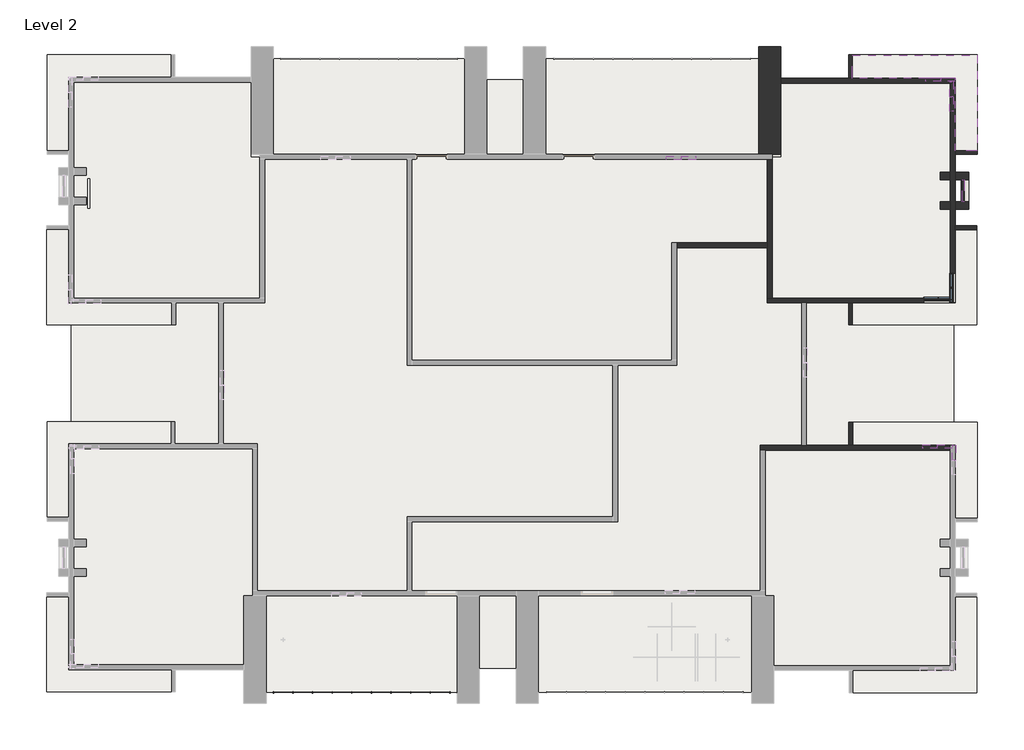
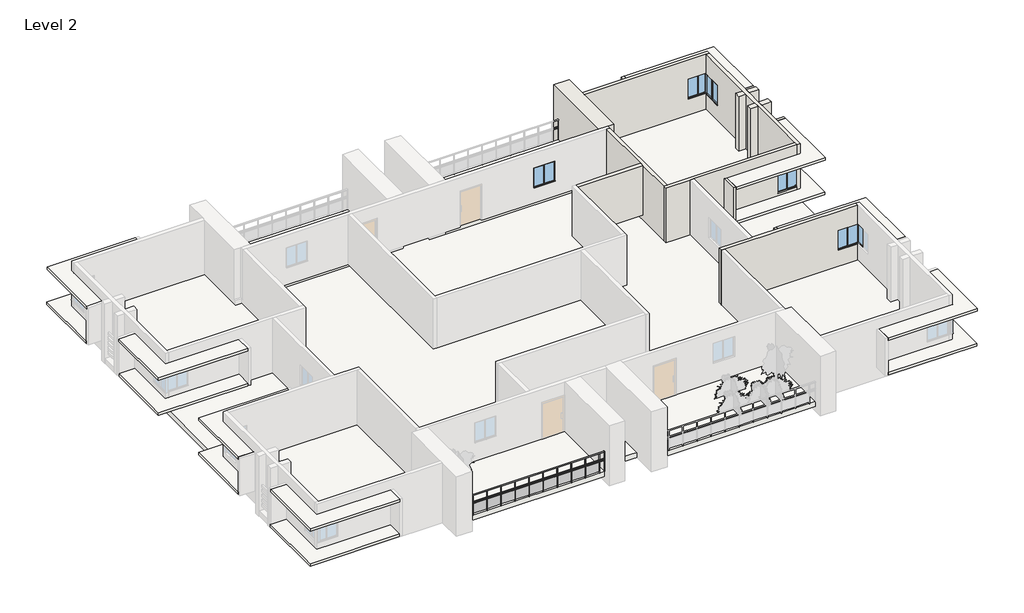
# One storey, part 3 of 4: 22 walls, 13 windows, 4 slabs, 1 railing.
"""IFC4 building model written with IfcOpenShell, lengths in millimetres."""

from ifc_helpers import new_model, si_unit, point, frame, origin, place, context, project, spatial, polyline, ellipse_curve, trimmed, outline, extrude, faceted_brep, transform, mapped, element, save
from ifc_brep_helpers import plane_surface, extruded_surface, advanced_brep
from components import window_20ff4747

model = new_model("IFC4")

# Units and contexts
model_context = context("Model", 3, world=origin())
ifc_project = project(units=[si_unit("LENGTHUNIT", "METRE", prefix="MILLI")], contexts=[model_context])

# Site, building, storey
site = spatial("IfcSite", under=ifc_project)
building = spatial("IfcBuilding", under=site)
storey = spatial("IfcBuildingStorey", under=building, Name="Level 2", Elevation=3048.0)

# Railing
placement = place(None, origin())
element("IfcRailing", 1, ObjectType="Glass Panel - Bottom Fill", at=placement, inside=storey, context=model_context, shape_type="SolidModel", body=[
    advanced_brep(
    [(-6704.9479335, -9342.282663, 4876.8), (-6704.9479335, -9418.482663, 4876.8), (1219.8520665, -9342.282663, 4876.8), (1219.8520665, -9418.482663, 4876.8)],
    [
        (0, 1, ellipse_curve(frame((-6704.9479335, -9380.382663, 4876.8), z_axis=(-1.0, 0.0, 0.0), x_axis=(0.0, -1.0, 0.0)), 38.1, 28.575)),
        (1, 0, ellipse_curve(frame((-6704.9479335, -9380.382663, 4876.8), z_axis=(-1.0, 0.0, 0.0), x_axis=(0.0, -1.0, 0.0)), 38.1, 28.575)),
        (2, 3, ellipse_curve(frame((1219.8520665, -9380.382663, 4876.8), z_axis=(1.0, 0.0, 0.0), x_axis=(0.0, -1.0, 0.0)), 38.1, 28.575)),
        (3, 2, ellipse_curve(frame((1219.8520665, -9380.382663, 4876.8), z_axis=(1.0, 0.0, 0.0), x_axis=(0.0, -1.0, 0.0)), 38.1, 28.575)),
        (0, 2),
        (3, 1),
    ],
    [
        plane_surface(frame((-6704.9479335, -9380.382663, 4876.8), z_axis=(-1.0, 0.0, 0.0), x_axis=(0.0, 1.0, 0.0))),
        plane_surface(frame((1219.8520665, -9380.382663, 4876.8), z_axis=(1.0, 0.0, 0.0), x_axis=(0.0, 1.0, 0.0))),
        extruded_surface(trimmed(ellipse_curve(frame((1219.8520665, -9380.382663, 4876.8), z_axis=(-1.0, 0.0, 0.0), x_axis=(0.0, -1.0, 0.0)), 38.1, 28.575), [point((1219.8520665, -9342.282663, 4876.8))], [point((1219.8520665, -9418.482663, 4876.8))], True, "CARTESIAN"), (-7924.799999999999, 0.0, 0.0), 7924.799999999999),
        extruded_surface(trimmed(ellipse_curve(frame((1219.8520665, -9380.382663, 4876.8), z_axis=(-1.0, 0.0, 0.0), x_axis=(0.0, -1.0, 0.0)), 38.1, 28.575), [point((1219.8520665, -9418.482663, 4876.8))], [point((1219.8520665, -9342.282663, 4876.8))], True, "CARTESIAN"), (-7924.799999999999, 0.0, 0.0), 7924.799999999999),
    ],
    [
        (0, [[1, 2]]),
        (1, [[3, 4]]),
        (2, [[-1, 5, -4, 6]]),
        (3, [[-2, -6, -3, -5]]),
    ],
),
    extrude(outline(polyline([(-6704.9479335, -9393.082663), (-6704.9479335, -9367.682663), (1219.8520665, -9367.682663), (1219.8520665, -9393.082663), (-6704.9479335, -9393.082663)])), frame((0.0, 0.0, 4457.7), z_axis=(0.0, 0.0, 1.0), x_axis=(1.0, 0.0, 0.0)), (0.0, 0.0, 1.0), 25.4),
    extrude(outline(polyline([(-6704.9479335, -9393.082663), (-6704.9479335, -9367.682663), (1219.8520665, -9367.682663), (1219.8520665, -9393.082663), (-6704.9479335, -9393.082663)])), frame((0.0, 0.0, 4356.1), z_axis=(0.0, 0.0, 1.0), x_axis=(1.0, 0.0, 0.0)), (0.0, 0.0, 1.0), 25.4),
    extrude(outline(polyline([(908.7020665, -9405.782663), (908.7020665, -9354.982663), (921.4020665, -9354.982663), (921.4020665, -9405.782663), (908.7020665, -9405.782663)])), frame((0.0, 0.0, 3657.6), z_axis=(0.0, 0.0, 1.0), x_axis=(1.0, 0.0, 0.0)), (0.0, 0.0, 1.0), 1190.4788223),
    extrude(outline(polyline([(102.2520665, -9373.847506), (915.0520665, -9373.847506), (915.0520665, -9380.197506), (102.2520665, -9380.197506), (102.2520665, -9373.847506)])), frame((0.0, 0.0, 3759.2), z_axis=(0.0, 0.0, 1.0), x_axis=(1.0, 0.0, 0.0)), (0.0, 0.0, 1.0), 596.9),
    extrude(outline(polyline([(95.9020665, -9405.782663), (95.9020665, -9354.982663), (108.6020665, -9354.982663), (108.6020665, -9405.782663), (95.9020665, -9405.782663)])), frame((0.0, 0.0, 3657.6), z_axis=(0.0, 0.0, 1.0), x_axis=(1.0, 0.0, 0.0)), (0.0, 0.0, 1.0), 1190.4788223),
    extrude(outline(polyline([(-710.5479335, -9373.847506), (102.2520665, -9373.847506), (102.2520665, -9380.197506), (-710.5479335, -9380.197506), (-710.5479335, -9373.847506)])), frame((0.0, 0.0, 3759.2), z_axis=(0.0, 0.0, 1.0), x_axis=(1.0, 0.0, 0.0)), (0.0, 0.0, 1.0), 596.9),
    extrude(outline(polyline([(-716.8979335, -9405.782663), (-716.8979335, -9354.982663), (-704.1979335, -9354.982663), (-704.1979335, -9405.782663), (-716.8979335, -9405.782663)])), frame((0.0, 0.0, 3657.6), z_axis=(0.0, 0.0, 1.0), x_axis=(1.0, 0.0, 0.0)), (0.0, 0.0, 1.0), 1190.4788223),
    extrude(outline(polyline([(-1523.3479335, -9373.847506), (-710.5479335, -9373.847506), (-710.5479335, -9380.197506), (-1523.3479335, -9380.197506), (-1523.3479335, -9373.847506)])), frame((0.0, 0.0, 3759.2), z_axis=(0.0, 0.0, 1.0), x_axis=(1.0, 0.0, 0.0)), (0.0, 0.0, 1.0), 596.9),
    extrude(outline(polyline([(-1529.6979335, -9405.782663), (-1529.6979335, -9354.982663), (-1516.9979335, -9354.982663), (-1516.9979335, -9405.782663), (-1529.6979335, -9405.782663)])), frame((0.0, 0.0, 3657.6), z_axis=(0.0, 0.0, 1.0), x_axis=(1.0, 0.0, 0.0)), (0.0, 0.0, 1.0), 1190.4788223),
    extrude(outline(polyline([(-2336.1479335, -9373.847506), (-1523.3479335, -9373.847506), (-1523.3479335, -9380.197506), (-2336.1479335, -9380.197506), (-2336.1479335, -9373.847506)])), frame((0.0, 0.0, 3759.2), z_axis=(0.0, 0.0, 1.0), x_axis=(1.0, 0.0, 0.0)), (0.0, 0.0, 1.0), 596.9),
    extrude(outline(polyline([(-2342.4979335, -9405.782663), (-2342.4979335, -9354.982663), (-2329.7979335, -9354.982663), (-2329.7979335, -9405.782663), (-2342.4979335, -9405.782663)])), frame((0.0, 0.0, 3657.6), z_axis=(0.0, 0.0, 1.0), x_axis=(1.0, 0.0, 0.0)), (0.0, 0.0, 1.0), 1190.4788223),
    extrude(outline(polyline([(-3148.9479335, -9373.847506), (-2336.1479335, -9373.847506), (-2336.1479335, -9380.197506), (-3148.9479335, -9380.197506), (-3148.9479335, -9373.847506)])), frame((0.0, 0.0, 3759.2), z_axis=(0.0, 0.0, 1.0), x_axis=(1.0, 0.0, 0.0)), (0.0, 0.0, 1.0), 596.9),
    extrude(outline(polyline([(-3155.2979335, -9405.782663), (-3155.2979335, -9354.982663), (-3142.5979335, -9354.982663), (-3142.5979335, -9405.782663), (-3155.2979335, -9405.782663)])), frame((0.0, 0.0, 3657.6), z_axis=(0.0, 0.0, 1.0), x_axis=(1.0, 0.0, 0.0)), (0.0, 0.0, 1.0), 1190.4788223),
    extrude(outline(polyline([(-3961.7479335, -9373.847506), (-3148.9479335, -9373.847506), (-3148.9479335, -9380.197506), (-3961.7479335, -9380.197506), (-3961.7479335, -9373.847506)])), frame((0.0, 0.0, 3759.2), z_axis=(0.0, 0.0, 1.0), x_axis=(1.0, 0.0, 0.0)), (0.0, 0.0, 1.0), 596.9),
    extrude(outline(polyline([(-3968.0979335, -9405.782663), (-3968.0979335, -9354.982663), (-3955.3979335, -9354.982663), (-3955.3979335, -9405.782663), (-3968.0979335, -9405.782663)])), frame((0.0, 0.0, 3657.6), z_axis=(0.0, 0.0, 1.0), x_axis=(1.0, 0.0, 0.0)), (0.0, 0.0, 1.0), 1190.4788223),
    extrude(outline(polyline([(-4774.5479335, -9373.847506), (-3961.7479335, -9373.847506), (-3961.7479335, -9380.197506), (-4774.5479335, -9380.197506), (-4774.5479335, -9373.847506)])), frame((0.0, 0.0, 3759.2), z_axis=(0.0, 0.0, 1.0), x_axis=(1.0, 0.0, 0.0)), (0.0, 0.0, 1.0), 596.9),
    extrude(outline(polyline([(-4780.8979335, -9405.782663), (-4780.8979335, -9354.982663), (-4768.1979335, -9354.982663), (-4768.1979335, -9405.782663), (-4780.8979335, -9405.782663)])), frame((0.0, 0.0, 3657.6), z_axis=(0.0, 0.0, 1.0), x_axis=(1.0, 0.0, 0.0)), (0.0, 0.0, 1.0), 1190.4788223),
    extrude(outline(polyline([(-5587.3479335, -9373.847506), (-4774.5479335, -9373.847506), (-4774.5479335, -9380.197506), (-5587.3479335, -9380.197506), (-5587.3479335, -9373.847506)])), frame((0.0, 0.0, 3759.2), z_axis=(0.0, 0.0, 1.0), x_axis=(1.0, 0.0, 0.0)), (0.0, 0.0, 1.0), 596.9),
    extrude(outline(polyline([(-5593.6979335, -9405.782663), (-5593.6979335, -9354.982663), (-5580.9979335, -9354.982663), (-5580.9979335, -9405.782663), (-5593.6979335, -9405.782663)])), frame((0.0, 0.0, 3657.6), z_axis=(0.0, 0.0, 1.0), x_axis=(1.0, 0.0, 0.0)), (0.0, 0.0, 1.0), 1190.4788223),
    extrude(outline(polyline([(-6400.1479335, -9373.847506), (-5587.3479335, -9373.847506), (-5587.3479335, -9380.197506), (-6400.1479335, -9380.197506), (-6400.1479335, -9373.847506)])), frame((0.0, 0.0, 3759.2), z_axis=(0.0, 0.0, 1.0), x_axis=(1.0, 0.0, 0.0)), (0.0, 0.0, 1.0), 596.9),
    extrude(outline(polyline([(-6406.4979335, -9405.782663), (-6406.4979335, -9354.982663), (-6393.7979335, -9354.982663), (-6393.7979335, -9405.782663), (-6406.4979335, -9405.782663)])), frame((0.0, 0.0, 3657.6), z_axis=(0.0, 0.0, 1.0), x_axis=(1.0, 0.0, 0.0)), (0.0, 0.0, 1.0), 1190.4788223),
    extrude(outline(polyline([(1207.1520665, -9389.907663), (1207.1520665, -9370.857663), (1226.2020665, -9370.857663), (1226.2020665, -9389.907663), (1207.1520665, -9389.907663)])), frame((0.0, 0.0, 3657.6), z_axis=(0.0, 0.0, 1.0), x_axis=(1.0, 0.0, 0.0)), (0.0, 0.0, 1.0), 1190.4788223),
    extrude(outline(polyline([(-6711.2979335, -9389.907663), (-6711.2979335, -9370.857663), (-6692.2479335, -9370.857663), (-6692.2479335, -9389.907663), (-6711.2979335, -9389.907663)])), frame((0.0, 0.0, 3657.6), z_axis=(0.0, 0.0, 1.0), x_axis=(1.0, 0.0, 0.0)), (0.0, 0.0, 1.0), 1190.4788223),
])

# Slabs
element("IfcSlab", 2, ObjectType="Generic - 2'", at=placement, inside=storey, context=model_context, shape_type="SweptSolid", body=[
    extrude(outline(polyline([(21793.8520665, 16006.5548886), (21793.8520665, -8377.4451114), (-14782.1479335, -8377.4451114), (-14782.1479335, 16006.5548886), (21793.8520665, 16006.5548886)])), frame((0.0, 0.0, 3048.0), z_axis=(0.0, 0.0, 1.0), x_axis=(1.0, 0.0, 0.0)), (0.0, 0.0, 1.0), 304.8),
])
element("IfcSlab", 3, ObjectType="Generic - 2' gray", at=placement, inside=storey, context=model_context, shape_type="SweptSolid", body=[
    extrude(outline(polyline([(13411.8520665, -5363.830811), (13411.8520665, -9380.382663), (4572.6520665, -9380.382663), (4572.6520665, -5363.830811), (13411.8520665, -5363.830811)])), frame((0.0, 0.0, 3352.8), z_axis=(0.0, 0.0, 1.0), x_axis=(1.0, 0.0, 0.0)), (0.0, 0.0, 1.0), 304.8),
    extrude(outline(polyline([(-6704.9479335, -5363.1461695), (1219.8520665, -5363.1461695), (1219.8520665, -9380.382663), (-6704.9479335, -9380.382663), (-6704.9479335, -5363.1461695)])), frame((0.0, 0.0, 3352.8), z_axis=(0.0, 0.0, 1.0), x_axis=(1.0, 0.0, 0.0)), (0.0, 0.0, 1.0), 304.8),
    extrude(outline(polyline([(13716.6520665, 12912.4705944), (4877.4520665, 12912.4705944), (4877.4520665, 16886.1559451), (13716.6520665, 16886.1559451), (13716.6520665, 12912.4705944)])), frame((0.0, 0.0, 3352.8), z_axis=(0.0, 0.0, 1.0), x_axis=(1.0, 0.0, 0.0)), (0.0, 0.0, 1.0), 304.8),
    extrude(outline(polyline([(-6400.1479335, 12912.4705944), (-6400.1479335, 16886.1559451), (1524.6520665, 16886.1559451), (1524.6520665, 12912.4705944), (-6400.1479335, 12912.4705944)])), frame((0.0, 0.0, 3352.8), z_axis=(0.0, 0.0, 1.0), x_axis=(1.0, 0.0, 0.0)), (0.0, 0.0, 1.0), 304.8),
])
element("IfcSlab", 4, ObjectType="Generic - 6\"", at=placement, inside=storey, context=model_context, shape_type="SweptSolid", body=[
    extrude(outline(polyline([(-10616.5479335, -9354.6604699), (-15798.1479335, -9354.6604699), (-15798.1479335, -5392.2604699), (-14883.7479335, -5392.2604699), (-14883.7479335, -8338.6604699), (-14883.7479335, -8440.2604699), (-10616.5479335, -8440.2604699), (-10616.5479335, -9354.6604699)])), frame((0.0, 0.0, 3810.0), z_axis=(0.0, 0.0, 1.0), x_axis=(1.0, 0.0, 0.0)), (0.0, 0.0, 1.0), 152.4),
    extrude(outline(polyline([(-10633.1034654, 1834.0395301), (-10633.1034654, 919.6395301), (-14883.7479335, 919.6395301), (-14883.7479335, -2128.3604699), (-15775.8097154, -2128.3604699), (-15775.8097154, 1834.0395301), (-10633.1034654, 1834.0395301)])), frame((0.0, 0.0, 3810.0), z_axis=(0.0, 0.0, 1.0), x_axis=(1.0, 0.0, 0.0)), (0.0, 0.0, 1.0), 152.4),
    extrude(outline(polyline([(-10616.5479335, 5846.5548886), (-15798.1479335, 5846.5548886), (-15798.1479335, 9808.9548886), (-14883.7479335, 9808.9548886), (-14883.7479335, 6862.5548886), (-14883.7479335, 6760.9548886), (-10616.5479335, 6760.9548886), (-10616.5479335, 5846.5548886)])), frame((0.0, 0.0, 3810.0), z_axis=(0.0, 0.0, 1.0), x_axis=(1.0, 0.0, 0.0)), (0.0, 0.0, 1.0), 152.4),
    extrude(outline(polyline([(-10633.1034654, 17035.2548886), (-10633.1034654, 16120.8548886), (-14883.7479335, 16120.8548886), (-14883.7479335, 13072.8548886), (-15775.8097154, 13072.8548886), (-15775.8097154, 17035.2548886), (-10633.1034654, 17035.2548886)])), frame((0.0, 0.0, 3810.0), z_axis=(0.0, 0.0, 1.0), x_axis=(1.0, 0.0, 0.0)), (0.0, 0.0, 1.0), 152.4),
    extrude(outline(polyline([(17590.1520665, 17035.2548886), (22771.7520665, 17035.2548886), (22771.7520665, 13072.8548886), (21857.3520665, 13072.8548886), (21857.3520665, 16019.2548886), (21857.3520665, 16070.0548886), (17590.1520665, 16070.0548886), (17590.1520665, 16120.8548886), (17590.1520665, 17035.2548886)])), frame((0.0, 0.0, 3810.0), z_axis=(0.0, 0.0, 1.0), x_axis=(1.0, 0.0, 0.0)), (0.0, 0.0, 1.0), 152.4),
    extrude(outline(polyline([(17606.7075984, 5846.5548886), (17606.7075984, 6760.9548886), (21857.3520665, 6760.9548886), (21857.3520665, 9808.9548886), (22749.4138484, 9808.9548886), (22749.4138484, 5846.5548886), (17606.7075984, 5846.5548886)])), frame((0.0, 0.0, 3810.0), z_axis=(0.0, 0.0, 1.0), x_axis=(1.0, 0.0, 0.0)), (0.0, 0.0, 1.0), 152.4),
    extrude(outline(polyline([(17590.1520665, 1807.9548886), (22771.7520665, 1807.9548886), (22771.7520665, -2154.4451114), (21857.3520665, -2154.4451114), (21857.3520665, 791.9548886), (21857.3520665, 893.5548886), (17590.1520665, 893.5548886), (17590.1520665, 1807.9548886)])), frame((0.0, 0.0, 3810.0), z_axis=(0.0, 0.0, 1.0), x_axis=(1.0, 0.0, 0.0)), (0.0, 0.0, 1.0), 152.4),
    extrude(outline(polyline([(17606.7075984, -9380.7451114), (17606.7075984, -8466.3451114), (21857.3520665, -8466.3451114), (21857.3520665, -5418.3451114), (22749.4138484, -5418.3451114), (22749.4138484, -9380.7451114), (17606.7075984, -9380.7451114)])), frame((0.0, 0.0, 3810.0), z_axis=(0.0, 0.0, 1.0), x_axis=(1.0, 0.0, 0.0)), (0.0, 0.0, 1.0), 152.4),
])
element("IfcSlab", 5, ObjectType="Generic - 6\"", at=placement, inside=storey, context=model_context, shape_type="SweptSolid", body=[
    extrude(outline(polyline([(-10617.0810044, -9363.7552779), (-15798.6810044, -9363.7552779), (-15798.6810044, -5401.3552779), (-14884.2810044, -5401.3552779), (-14884.2810044, -8347.7552779), (-14884.2810044, -8449.3552779), (-10617.0810044, -8449.3552779), (-10617.0810044, -9363.7552779)])), frame((0.0, 0.0, 5943.6), z_axis=(0.0, 0.0, 1.0), x_axis=(1.0, 0.0, 0.0)), (0.0, 0.0, 1.0), 152.4),
    extrude(outline(polyline([(-10633.6365363, 1824.9447221), (-10633.6365363, 910.5447221), (-14884.2810044, 910.5447221), (-14884.2810044, -2137.4552779), (-15776.3427863, -2137.4552779), (-15776.3427863, 1824.9447221), (-10633.6365363, 1824.9447221)])), frame((0.0, 0.0, 5943.6), z_axis=(0.0, 0.0, 1.0), x_axis=(1.0, 0.0, 0.0)), (0.0, 0.0, 1.0), 152.4),
    extrude(outline(polyline([(-10617.0810044, 5837.4600805), (-15798.6810044, 5837.4600805), (-15798.6810044, 9799.8600805), (-14884.2810044, 9799.8600805), (-14884.2810044, 6853.4600805), (-14884.2810044, 6751.8600805), (-10617.0810044, 6751.8600805), (-10617.0810044, 5837.4600805)])), frame((0.0, 0.0, 5943.6), z_axis=(0.0, 0.0, 1.0), x_axis=(1.0, 0.0, 0.0)), (0.0, 0.0, 1.0), 152.4),
    extrude(outline(polyline([(-10633.6365363, 17026.1600805), (-10633.6365363, 16111.7600805), (-14884.2810044, 16111.7600805), (-14884.2810044, 13063.7600805), (-15776.3427863, 13063.7600805), (-15776.3427863, 17026.1600805), (-10633.6365363, 17026.1600805)])), frame((0.0, 0.0, 5943.6), z_axis=(0.0, 0.0, 1.0), x_axis=(1.0, 0.0, 0.0)), (0.0, 0.0, 1.0), 152.4),
    extrude(outline(polyline([(17589.6189956, 17026.1600805), (22771.2189956, 17026.1600805), (22771.2189956, 13063.7600805), (21856.8189956, 13063.7600805), (21856.8189956, 16010.1600805), (21856.8189956, 16060.9600805), (17589.6189956, 16060.9600805), (17589.6189956, 16111.7600805), (17589.6189956, 17026.1600805)])), frame((0.0, 0.0, 5943.6), z_axis=(0.0, 0.0, 1.0), x_axis=(1.0, 0.0, 0.0)), (0.0, 0.0, 1.0), 152.4),
    extrude(outline(polyline([(17606.1745274, 5837.4600805), (17606.1745274, 6751.8600805), (21856.8189956, 6751.8600805), (21856.8189956, 9799.8600805), (22748.8807774, 9799.8600805), (22748.8807774, 5837.4600805), (17606.1745274, 5837.4600805)])), frame((0.0, 0.0, 5943.6), z_axis=(0.0, 0.0, 1.0), x_axis=(1.0, 0.0, 0.0)), (0.0, 0.0, 1.0), 152.4),
    extrude(outline(polyline([(17589.6189956, 1798.8600805), (22771.2189956, 1798.8600805), (22771.2189956, -2163.5399195), (21856.8189956, -2163.5399195), (21856.8189956, 782.8600805), (21856.8189956, 884.4600805), (17589.6189956, 884.4600805), (17589.6189956, 1798.8600805)])), frame((0.0, 0.0, 5943.6), z_axis=(0.0, 0.0, 1.0), x_axis=(1.0, 0.0, 0.0)), (0.0, 0.0, 1.0), 152.4),
    extrude(outline(polyline([(17606.1745274, -9389.8399195), (17606.1745274, -8475.4399195), (21856.8189956, -8475.4399195), (21856.8189956, -5427.4399195), (22748.8807774, -5427.4399195), (22748.8807774, -9389.8399195), (17606.1745274, -9389.8399195)])), frame((0.0, 0.0, 5943.6), z_axis=(0.0, 0.0, 1.0), x_axis=(1.0, 0.0, 0.0)), (0.0, 0.0, 1.0), 152.4),
])

# Walls
element("IfcWall", 6, ObjectType="Generic - 1'", at=placement, inside=storey, context=model_context, shape_type="Brep", body=[
    faceted_brep([(21857.3520665, 11871.0705944, 3048.0), (22100.7496596, 11871.0705944, 3048.0), (22405.5496596, 11871.0705944, 3048.0), (22405.5496596, 11871.0705944, 3352.8), (22405.5496596, 11871.0705944, 6705.6), (21857.3520665, 11871.0705944, 6705.6), (21857.3520665, 12175.8705944, 3048.0), (21857.3520665, 12175.8705944, 6705.6), (22405.5496596, 12175.8705944, 6705.6), (22405.5496596, 12175.8705944, 3048.0)], [[[0, 1, 2, 3, 4, 5]], [[6, 7, 8, 9]], [[2, 1, 0, 6, 9]], [[5, 4, 8, 7]], [[0, 5, 7, 6]], [[4, 3, 2, 9, 8]]]),
])
element("IfcWall", 7, ObjectType="Generic - 1'", at=placement, inside=storey, context=model_context, shape_type="SweptSolid", body=[
    extrude(outline(polyline([(21235.7605971, 12175.8705944), (21654.1520665, 12175.8705944), (21654.1520665, 11871.0705944), (21235.7605971, 11871.0705944), (21235.7605971, 12175.8705944)])), frame((0.0, 0.0, 3048.0), z_axis=(0.0, 0.0, 1.0), x_axis=(1.0, 0.0, 0.0)), (0.0, 0.0, 1.0), 3657.6),
])
element("IfcWall", 8, ObjectType="Generic - 1'", at=placement, inside=storey, context=model_context, shape_type="Brep", body=[
    faceted_brep([(21857.3520665, 10651.8705944, 3048.0), (22405.5496596, 10651.8705944, 3048.0), (22405.5496596, 10651.8705944, 6705.6), (21857.3520665, 10651.8705944, 6705.6), (21857.3520665, 10956.6705944, 3048.0), (21857.3520665, 10956.6705944, 6705.6), (22405.5496596, 10956.6705944, 6705.6), (22405.5496596, 10956.6705944, 3352.8), (22405.5496596, 10956.6705944, 3048.0), (22100.7496596, 10956.6705944, 3048.0)], [[[0, 1, 2, 3]], [[4, 5, 6, 7, 8, 9]], [[1, 0, 4, 9, 8]], [[3, 2, 6, 5]], [[0, 3, 5, 4]], [[2, 1, 8, 7, 6]]]),
])
element("IfcWall", 9, ObjectType="Generic - 1'", at=placement, inside=storey, context=model_context, shape_type="SweptSolid", body=[
    extrude(outline(polyline([(21235.7605971, 10956.6705944), (21654.1520665, 10956.6705944), (21654.1520665, 10651.8705944), (21235.7605971, 10651.8705944), (21235.7605971, 10956.6705944)])), frame((0.0, 0.0, 3048.0), z_axis=(0.0, 0.0, 1.0), x_axis=(1.0, 0.0, 0.0)), (0.0, 0.0, 1.0), 3657.6),
])
element("IfcWall", 10, ObjectType="Generic - 2'", at=placement, inside=storey, context=model_context, shape_type="SweptSolid", body=[
    extrude(outline(polyline([(22100.7496596, 10956.6705944), (22100.7496596, 11871.0705944), (22405.5496596, 11871.0705944), (22405.5496596, 10956.6705944), (22100.7496596, 10956.6705944)])), frame((0.0, 0.0, 3048.0), z_axis=(0.0, 0.0, 1.0), x_axis=(1.0, 0.0, 0.0)), (0.0, 0.0, 1.0), 304.8),
])
element("IfcWall", 11, ObjectType="Generic - 3'", at=placement, inside=storey, context=model_context, shape_type="Brep", body=[
    faceted_brep([(14631.0520665, 12810.8705944, 3048.0), (14631.0520665, 15866.8548886, 3048.0), (14631.0520665, 16070.0548886, 3048.0), (14631.0520665, 17382.8705944, 3048.0), (14631.0520665, 17382.8705944, 6705.6), (14631.0520665, 16070.0548886, 6705.6), (14631.0520665, 15866.8548886, 6705.6), (14631.0520665, 12912.4705944, 6705.6), (14631.0520665, 12912.4705944, 3657.6), (14631.0520665, 12810.8705944, 3657.6), (13716.6520665, 12810.8705944, 3048.0), (13716.6520665, 12810.8705944, 3657.6), (13716.6520665, 12912.4705944, 3657.6), (13716.6520665, 12912.4705944, 6705.6), (13716.6520665, 17382.8705944, 6705.6), (13716.6520665, 17382.8705944, 3048.0), (14275.4520665, 12810.8705944, 3048.0), (14072.2520665, 12810.8705944, 3048.0), (14275.4520665, 12912.4705944, 6705.6), (14275.4520665, 12810.8705944, 3657.6), (14072.2520665, 12810.8705944, 3657.6), (14275.4520665, 12912.4705944, 3657.6)], [[[0, 1, 2, 3, 4, 5, 6, 7, 8, 9]], [[10, 11, 12, 13, 14, 15]], [[3, 2, 1, 0, 16, 17, 10, 15]], [[4, 3, 15, 14]], [[7, 6, 5, 4, 14, 13, 18]], [[0, 9, 19, 20, 11, 10, 17, 16]], [[8, 21, 12, 11, 20, 19, 9]], [[8, 7, 18, 13, 12, 21]]]),
])
element("IfcWall", 12, ObjectType="Generic - 5\"", at=placement, inside=storey, context=model_context, shape_type="SweptSolid", body=[
    extrude(outline(polyline([(22145.9857703, 10956.6705944), (22145.9857703, 11871.0705944), (22222.1857703, 11871.0705944), (22222.1857703, 10956.6705944), (22145.9857703, 10956.6705944)])), frame((0.0, 0.0, 3581.4), z_axis=(0.0, 0.0, 1.0), x_axis=(1.0, 0.0, 0.0)), (0.0, 0.0, 1.0), 152.8735856),
])
element("IfcWall", 13, ObjectType="Generic - 5\"", at=placement, inside=storey, context=model_context, shape_type="SweptSolid", body=[
    extrude(outline(polyline([(22145.9857703, 10956.6705944), (22145.9857703, 11871.0705944), (22222.1857703, 11871.0705944), (22222.1857703, 10956.6705944), (22145.9857703, 10956.6705944)])), frame((0.0, 0.0, 3860.8), z_axis=(0.0, 0.0, 1.0), x_axis=(1.0, 0.0, 0.0)), (0.0, 0.0, 1.0), 152.8735856),
])
element("IfcWall", 14, ObjectType="Generic - 5\"", at=placement, inside=storey, context=model_context, shape_type="SweptSolid", body=[
    extrude(outline(polyline([(22145.9857703, 10956.6705944), (22145.9857703, 11871.0705944), (22222.1857703, 11871.0705944), (22222.1857703, 10956.6705944), (22145.9857703, 10956.6705944)])), frame((0.0, 0.0, 4165.6), z_axis=(0.0, 0.0, 1.0), x_axis=(1.0, 0.0, 0.0)), (0.0, 0.0, 1.0), 152.8735856),
])
element("IfcWall", 15, ObjectType="Generic - 5\"", at=placement, inside=storey, context=model_context, shape_type="SweptSolid", body=[
    extrude(outline(polyline([(22145.9857703, 10956.6705944), (22145.9857703, 11871.0705944), (22222.1857703, 11871.0705944), (22222.1857703, 10956.6705944), (22145.9857703, 10956.6705944)])), frame((0.0, 0.0, 4470.4), z_axis=(0.0, 0.0, 1.0), x_axis=(1.0, 0.0, 0.0)), (0.0, 0.0, 1.0), 152.8735856),
])
element("IfcWall", 16, ObjectType="Generic - 5\"", at=placement, inside=storey, context=model_context, shape_type="SweptSolid", body=[
    extrude(outline(polyline([(22145.9857703, 10956.6705944), (22145.9857703, 11871.0705944), (22222.1857703, 11871.0705944), (22222.1857703, 10956.6705944), (22145.9857703, 10956.6705944)])), frame((0.0, 0.0, 4749.8), z_axis=(0.0, 0.0, 1.0), x_axis=(1.0, 0.0, 0.0)), (0.0, 0.0, 1.0), 152.8735856),
])
element("IfcWall", 17, ObjectType="Generic - 6\"", at=placement, inside=storey, context=model_context, shape_type="SweptSolid", body=[
    extrude(outline(polyline([(22771.7520665, 12914.1048886), (21857.3520665, 12914.1048886), (21857.3520665, 13066.5048886), (22771.7520665, 13066.5048886), (22771.7520665, 12914.1048886)])), frame((0.0, 0.0, 3810.0), z_axis=(0.0, 0.0, 1.0), x_axis=(1.0, 0.0, 0.0)), (0.0, 0.0, 1.0), 2286.0),
])
element("IfcWall", 18, ObjectType="Generic - 6\"", at=placement, inside=storey, context=model_context, shape_type="SweptSolid", body=[
    extrude(outline(polyline([(17590.1520665, 17035.2548886), (17590.1520665, 16070.0548886), (17437.7520665, 16070.0548886), (17437.7520665, 17035.2548886), (17590.1520665, 17035.2548886)])), frame((0.0, 0.0, 3810.0), z_axis=(0.0, 0.0, 1.0), x_axis=(1.0, 0.0, 0.0)), (0.0, 0.0, 1.0), 2286.0),
])
element("IfcWall", 19, ObjectType="Generic - 6\"", at=placement, inside=storey, context=model_context, shape_type="SweptSolid", body=[
    extrude(outline(polyline([(22748.8807774, 9799.8600805), (21857.3520665, 9799.8600805), (21857.3520665, 9952.2600805), (22748.8807774, 9952.2600805), (22748.8807774, 9799.8600805)])), frame((0.0, 0.0, 3810.0), z_axis=(0.0, 0.0, 1.0), x_axis=(1.0, 0.0, 0.0)), (0.0, 0.0, 1.0), 2286.0),
])
element("IfcWall", 20, ObjectType="Generic - 6\"", at=placement, inside=storey, context=model_context, shape_type="SweptSolid", body=[
    extrude(outline(polyline([(17441.6075984, 5850.1600805), (17441.6075984, 6760.9548886), (17594.0075984, 6760.9548886), (17594.0075984, 5850.1600805), (17441.6075984, 5850.1600805)])), frame((0.0, 0.0, 3810.0), z_axis=(0.0, 0.0, 1.0), x_axis=(1.0, 0.0, 0.0)), (0.0, 0.0, 1.0), 2286.0),
])
element("IfcWall", 21, ObjectType="Generic - 6\"", at=placement, inside=storey, context=model_context, shape_type="SweptSolid", body=[
    extrude(outline(polyline([(17595.9689956, 1807.9548886), (17595.9689956, 868.1548886), (17443.5689956, 868.1548886), (17443.5689956, 1807.9548886), (17595.9689956, 1807.9548886)])), frame((0.0, 0.0, 3810.0), z_axis=(0.0, 0.0, 1.0), x_axis=(1.0, 0.0, 0.0)), (0.0, 0.0, 1.0), 2286.0),
])
element("IfcWall", 22, ObjectType="Generic - 8\"", at=placement, inside=storey, context=model_context, shape_type="SweptSolid", body=[
    extrude(outline(polyline([(14072.2520665, 9051.6705944), (10313.0520665, 9051.6705944), (10313.0520665, 9254.8705944), (14072.2520665, 9254.8705944), (14072.2520665, 9051.6705944)])), frame((0.0, 0.0, 3657.6), z_axis=(0.0, 0.0, 1.0), x_axis=(1.0, 0.0, 0.0)), (0.0, 0.0, 1.0), 3048.0),
])
element("IfcWall", 23, ObjectType="Generic - 8\" gray", at=placement, inside=storey, context=model_context, shape_type="Brep", body=[
    faceted_brep([(21857.3520665, 16070.0548886, 3048.0), (14631.0520665, 16070.0548886, 3048.0), (14631.0520665, 16070.0548886, 6705.6), (21857.3520665, 16070.0548886, 6705.6), (20634.9770665, 16070.0548886, 4320.2804451), (21854.1770665, 16070.0548886, 4320.2804451), (21854.1770665, 16070.0548886, 5539.4804451), (20634.9770665, 16070.0548886, 5539.4804451), (14631.0520665, 15866.8548886, 3048.0), (21654.1520665, 15866.8548886, 3048.0), (21857.3520665, 15866.8548886, 3048.0), (21857.3520665, 15866.8548886, 4302.1280277), (21857.3520665, 15866.8548886, 5521.3280277), (21857.3520665, 15866.8548886, 6705.6), (21654.1520665, 15866.8548886, 6705.6), (14631.0520665, 15866.8548886, 6705.6), (20634.9770665, 15866.8548886, 5539.4804451), (21854.1770665, 15866.8548886, 5539.4804451), (21854.1770665, 15866.8548886, 4320.2804451), (20634.9770665, 15866.8548886, 4320.2804451)], [[[0, 1, 2, 3], [4, 5, 6, 7]], [[8, 9, 10, 11, 12, 13, 14, 15], [16, 17, 18, 19]], [[1, 0, 10, 9, 8]], [[3, 2, 15, 14, 13]], [[0, 3, 13, 12, 11, 10]], [[2, 1, 8, 15]], [[18, 17, 6, 5]], [[18, 5, 4, 19]], [[16, 7, 6, 17]], [[19, 4, 7, 16]]]),
])
element("IfcWall", 24, ObjectType="Generic - 8\" gray", at=placement, inside=storey, context=model_context, shape_type="Brep", body=[
    faceted_brep([(21857.3520665, 6760.9548886, 3048.0), (21857.3520665, 10651.8705944, 3048.0), (21857.3520665, 10956.6705944, 3048.0), (21857.3520665, 11871.0705944, 3048.0), (21857.3520665, 12175.8705944, 3048.0), (21857.3520665, 15866.8548886, 3048.0), (21857.3520665, 15866.8548886, 4302.1280277), (21857.3520665, 14696.4442594, 4302.1280277), (21857.3520665, 14696.4442594, 5521.3280277), (21857.3520665, 15866.8548886, 5521.3280277), (21857.3520665, 15866.8548886, 6705.6), (21857.3520665, 12175.8705944, 6705.6), (21857.3520665, 11871.0705944, 6705.6), (21857.3520665, 10956.6705944, 6705.6), (21857.3520665, 10651.8705944, 6705.6), (21857.3520665, 6760.9548886, 6705.6), (21857.3520665, 7997.1026284, 4155.0947232), (21857.3520665, 6777.9026284, 4155.0947232), (21857.3520665, 6777.9026284, 5374.2947232), (21857.3520665, 7997.1026284, 5374.2947232), (21654.1520665, 15866.8548886, 3048.0), (21654.1520665, 12175.8705944, 3048.0), (21654.1520665, 11871.0705944, 3048.0), (21654.1520665, 10956.6705944, 3048.0), (21654.1520665, 10651.8705944, 3048.0), (21654.1520665, 6964.1548886, 3048.0), (21654.1520665, 6760.9548886, 3048.0), (21654.1520665, 6760.9548886, 4105.9450479), (21654.1520665, 6760.9548886, 5325.1450479), (21654.1520665, 6760.9548886, 6705.6), (21654.1520665, 6964.1548886, 6705.6), (21654.1520665, 10651.8705944, 6705.6), (21654.1520665, 10956.6705944, 6705.6), (21654.1520665, 11871.0705944, 6705.6), (21654.1520665, 12175.8705944, 6705.6), (21654.1520665, 15866.8548886, 6705.6), (21654.1520665, 15866.8548886, 5521.3280277), (21654.1520665, 14696.4442594, 5521.3280277), (21654.1520665, 14696.4442594, 4302.1280277), (21654.1520665, 15866.8548886, 4302.1280277), (21654.1520665, 6777.9026284, 4155.0947232), (21654.1520665, 7997.1026284, 4155.0947232), (21654.1520665, 7997.1026284, 5374.2947232), (21654.1520665, 6777.9026284, 5374.2947232)], [[[0, 1, 2, 3, 4, 5, 6, 7, 8, 9, 10, 11, 12, 13, 14, 15], [16, 17, 18, 19]], [[20, 21, 22, 23, 24, 25, 26, 27, 28, 29, 30, 31, 32, 33, 34, 35, 36, 37, 38, 39], [40, 41, 42, 43]], [[5, 4, 3, 2, 1, 0, 26, 25, 24, 23, 22, 21, 20]], [[15, 14, 13, 12, 11, 10, 35, 34, 33, 32, 31, 30, 29]], [[0, 15, 29, 28, 27, 26]], [[5, 20, 39, 6]], [[35, 10, 9, 36]], [[38, 7, 6, 39]], [[8, 7, 38, 37]], [[8, 37, 36, 9]], [[16, 41, 40, 17]], [[18, 43, 42, 19]], [[19, 42, 41, 16]], [[43, 18, 17, 40]]]),
])
element("IfcWall", 25, ObjectType="Generic - 8\" gray", at=placement, inside=storey, context=model_context, shape_type="Brep", body=[
    faceted_brep([(14072.2520665, 6760.9548886, 3048.0), (15481.9520665, 6760.9548886, 3048.0), (15685.1520665, 6760.9548886, 3048.0), (21654.1520665, 6760.9548886, 3048.0), (21654.1520665, 6760.9548886, 4105.9450479), (20541.6213445, 6760.9548886, 4105.9450479), (20541.6213445, 6760.9548886, 5325.1450479), (21654.1520665, 6760.9548886, 5325.1450479), (21654.1520665, 6760.9548886, 6705.6), (15685.1520665, 6760.9548886, 6705.6), (15481.9520665, 6760.9548886, 6705.6), (14072.2520665, 6760.9548886, 6705.6), (21654.1520665, 6964.1548886, 3048.0), (14275.4520665, 6964.1548886, 3048.0), (14072.2520665, 6964.1548886, 3048.0), (14072.2520665, 6964.1548886, 6705.6), (14275.4520665, 6964.1548886, 6705.6), (21654.1520665, 6964.1548886, 6705.6), (21654.1520665, 6964.1548886, 5325.1450479), (20541.6213445, 6964.1548886, 5325.1450479), (20541.6213445, 6964.1548886, 4105.9450479), (21654.1520665, 6964.1548886, 4105.9450479)], [[[0, 1, 2, 3, 4, 5, 6, 7, 8, 9, 10, 11]], [[12, 13, 14, 15, 16, 17, 18, 19, 20, 21]], [[3, 2, 1, 0, 14, 13, 12]], [[11, 10, 9, 8, 17, 16, 15]], [[3, 12, 21, 4]], [[17, 8, 7, 18]], [[0, 11, 15, 14]], [[4, 21, 20, 5]], [[6, 5, 20, 19]], [[6, 19, 18, 7]]]),
])
element("IfcWall", 26, ObjectType="Generic - 8\" gray", at=placement, inside=storey, context=model_context, shape_type="Brep", body=[
    faceted_brep([(13767.4520665, 664.9548886, 3048.0), (13970.6520665, 664.9548886, 3048.0), (21654.1520665, 664.9548886, 3048.0), (21654.1520665, 664.9548886, 4320.2804451), (20505.783383, 664.9548886, 4320.2804451), (20505.783383, 664.9548886, 5539.4804451), (21654.1520665, 664.9548886, 5539.4804451), (21654.1520665, 664.9548886, 6705.6), (13970.6520665, 664.9548886, 6705.6), (13767.4520665, 664.9548886, 6705.6), (21654.1520665, 868.1548886, 3048.0), (15685.1520665, 868.1548886, 3048.0), (15481.9520665, 868.1548886, 3048.0), (13767.4520665, 868.1548886, 3048.0), (13767.4520665, 868.1548886, 6705.6), (15481.9520665, 868.1548886, 6705.6), (15685.1520665, 868.1548886, 6705.6), (21654.1520665, 868.1548886, 6705.6), (21654.1520665, 868.1548886, 5539.4804451), (20505.783383, 868.1548886, 5539.4804451), (20505.783383, 868.1548886, 4320.2804451), (21654.1520665, 868.1548886, 4320.2804451), (21654.1520665, 859.364485, 4320.2804451), (21654.1520665, 859.364485, 5539.4804451)], [[[0, 1, 2, 3, 4, 5, 6, 7, 8, 9]], [[10, 11, 12, 13, 14, 15, 16, 17, 18, 19, 20, 21]], [[2, 1, 0, 13, 12, 11, 10]], [[9, 8, 7, 17, 16, 15, 14]], [[2, 10, 21, 22, 3]], [[17, 7, 6, 23, 18]], [[0, 9, 14, 13]], [[3, 22, 21, 20, 4]], [[5, 4, 20, 19]], [[5, 19, 18, 23, 6]]]),
])
element("IfcWall", 27, ObjectType="Generic - 8\" gray", at=placement, inside=storey, context=model_context, shape_type="Brep", body=[
    faceted_brep([(14275.4520665, 6964.1548886, 3048.0), (14275.4520665, 12810.8705944, 3048.0), (14275.4520665, 12810.8705944, 3657.6), (14275.4520665, 12709.2705944, 3657.6), (14275.4520665, 12709.2705944, 6705.6), (14275.4520665, 6964.1548886, 6705.6), (14072.2520665, 6964.1548886, 3048.0), (14072.2520665, 6964.1548886, 6705.6), (14072.2520665, 9051.6705944, 6705.6), (14072.2520665, 9254.8705944, 6705.6), (14072.2520665, 12709.2705944, 6705.6), (14072.2520665, 12709.2705944, 3657.6), (14072.2520665, 12810.8705944, 3657.6), (14072.2520665, 12810.8705944, 3048.0)], [[[0, 1, 2, 3, 4, 5]], [[6, 7, 8, 9, 10, 11, 12, 13]], [[1, 0, 6, 13]], [[5, 4, 10, 9, 8, 7]], [[0, 5, 7, 6]], [[2, 1, 13, 12]], [[11, 3, 2, 12]], [[4, 3, 11, 10]]]),
])

# Windows
window_shape = window_20ff4747(model_context)
element("IfcWindow", 28, ObjectType="Instance - Fixed : 24\" x 48\"", at=placement, inside=storey, context=model_context, shape_type="MappedRepresentation", body=[
    mapped(window_shape, transform((21587.4770665, 15968.4548886, 3405.8804451), x_axis=(1.0, 0.0, 0.0), y_axis=(0.0, 1.0, 0.0), z_axis=(0.0, 0.0, 1.0))),
])
element("IfcWindow", 29, ObjectType="Instance - Fixed : 24\" x 48\"", at=placement, inside=storey, context=model_context, shape_type="MappedRepresentation", body=[
    mapped(window_shape, transform((20977.8770665, 15968.4548886, 3405.8804451), x_axis=(1.0, 0.0, 0.0), y_axis=(0.0, 1.0, 0.0), z_axis=(0.0, 0.0, 1.0))),
])
element("IfcWindow", 30, ObjectType="Instance - Fixed : 24\" x 48\"", at=placement, inside=storey, context=model_context, shape_type="MappedRepresentation", body=[
    mapped(window_shape, transform((21755.7520665, 15648.9442594, 3387.7280277), x_axis=(0.0, 1.0, 0.0), y_axis=(-1.0, 0.0, 0.0), z_axis=(0.0, 0.0, 1.0))),
])
element("IfcWindow", 31, ObjectType="Instance - Fixed : 24\" x 48\"", at=placement, inside=storey, context=model_context, shape_type="MappedRepresentation", body=[
    mapped(window_shape, transform((21755.7520665, 15039.3442594, 3387.7280277), x_axis=(0.0, 1.0, 0.0), y_axis=(-1.0, 0.0, 0.0), z_axis=(0.0, 0.0, 1.0))),
])
element("IfcWindow", 32, ObjectType="Instance - Fixed : 24\" x 48\"", at=placement, inside=storey, context=model_context, shape_type="MappedRepresentation", body=[
    mapped(window_shape, transform((21458.283383, 766.5548886, 3405.8804451), x_axis=(1.0, 0.0, 0.0), y_axis=(0.0, 1.0, 0.0), z_axis=(0.0, 0.0, 1.0))),
])
element("IfcWindow", 33, ObjectType="Instance - Fixed : 24\" x 48\"", at=placement, inside=storey, context=model_context, shape_type="MappedRepresentation", body=[
    mapped(window_shape, transform((20848.683383, 766.5548886, 3405.8804451), x_axis=(1.0, 0.0, 0.0), y_axis=(0.0, 1.0, 0.0), z_axis=(0.0, 0.0, 1.0))),
])
element("IfcWindow", 34, ObjectType="Instance - Fixed : 24\" x 48\"", at=placement, inside=storey, context=model_context, shape_type="MappedRepresentation", body=[
    mapped(window_shape, transform((21755.7520665, 516.464485, 3405.8804451), x_axis=(0.0, -1.0, 0.0), y_axis=(1.0, 0.0, 0.0), z_axis=(0.0, 0.0, 1.0))),
])
element("IfcWindow", 35, ObjectType="Instance - Fixed : 24\" x 48\"", at=placement, inside=storey, context=model_context, shape_type="MappedRepresentation", body=[
    mapped(window_shape, transform((21755.7520665, 7730.4026284, 3240.6947232), x_axis=(0.0, 1.0, 0.0), y_axis=(-1.0, 0.0, 0.0), z_axis=(0.0, 0.0, 1.0))),
])
element("IfcWindow", 36, ObjectType="Instance - Fixed : 24\" x 48\"", at=placement, inside=storey, context=model_context, shape_type="MappedRepresentation", body=[
    mapped(window_shape, transform((21755.7520665, 7120.8026284, 3240.6947232), x_axis=(0.0, 1.0, 0.0), y_axis=(-1.0, 0.0, 0.0), z_axis=(0.0, 0.0, 1.0))),
])
element("IfcWindow", 37, ObjectType="Instance - Fixed : 24\" x 48\"", at=placement, inside=storey, context=model_context, shape_type="MappedRepresentation", body=[
    mapped(window_shape, transform((21494.1213445, 6862.5548886, 3191.5450479), x_axis=(1.0, 0.0, 0.0), y_axis=(0.0, 1.0, 0.0), z_axis=(0.0, 0.0, 1.0))),
])
element("IfcWindow", 38, ObjectType="Instance - Fixed : 24\" x 48\"", at=placement, inside=storey, context=model_context, shape_type="MappedRepresentation", body=[
    mapped(window_shape, transform((20884.5213445, 6862.5548886, 3191.5450479), x_axis=(1.0, 0.0, 0.0), y_axis=(0.0, 1.0, 0.0), z_axis=(0.0, 0.0, 1.0))),
])
element("IfcWindow", 39, ObjectType="Instance - Fixed : 24\" x 48\"", at=placement, inside=storey, context=model_context, shape_type="MappedRepresentation", body=[
    mapped(window_shape, transform((10149.6500799, 12810.8705944, 3662.4873953), x_axis=(-1.0, 0.0, 0.0), y_axis=(0.0, -1.0, 0.0), z_axis=(0.0, 0.0, 1.0))),
])
element("IfcWindow", 40, ObjectType="Instance - Fixed : 24\" x 48\"", at=placement, inside=storey, context=model_context, shape_type="MappedRepresentation", body=[
    mapped(window_shape, transform((10759.2500799, 12810.8705944, 3662.4873953), x_axis=(-1.0, 0.0, 0.0), y_axis=(0.0, -1.0, 0.0), z_axis=(0.0, 0.0, 1.0))),
])

save(model, "model.ifc")

# Revit data of these elements
# Type "Glass Panel - Bottom Fill"
#   Assembly Code = "C2010400"
#   built-in parameter 1008612 = 0.0416667 (stored number, unit not read)
#   built-in parameter 1008611 = 0.0416667 (stored number, unit not read)
#   built-in parameter 1008609 = 0.333333 (stored number, unit not read)
#   built-in parameter 1008604 = 0.166667 (stored number, unit not read)
#   built-in parameter 1008603 = 0.166667 (stored number, unit not read)
#   Railing Height = 4' - 0"
#   built-in parameter 1008630 = 2
#   built-in parameter 1008610 = 2
#   built-in parameter 1008618 = Baluster - Square : 3/4"
# Type "Generic - 2'"
#   Assembly Code = "B1010"
#   Function = 0
#   Layers, outside or top first: 1' - 0" "Metal - Painted - Grey" (function 1)
# Type "Generic - 2' gray"
#   Assembly Code = "B1010"
#   Function = 0
#   Layers, outside or top first: 1' - 0" "Rigid insulation" (function 1)
# Type "Generic - 6\""
#   Assembly Code = "B1010"
#   Function = 0
#   Layers, outside or top first: 0' - 6" "Metal - Painted - Grey" (function 1)
# Type "Generic - 1'"
#   Assembly Code = "B2010"
#   Layers, outside or top first: 1' - 0" "Metal - Painted - Grey" (function 1)
# Type "Generic - 2'"
#   Assembly Code = "B2010"
#   Layers, outside or top first: 1' - 0" "Metal - Painted - Grey" (function 1)
# Type "Generic - 3'"
#   Assembly Code = "B2010"
#   Layers, outside or top first: 3' - 0" "Metal - Painted - Grey" (function 1)
# Type "Generic - 5\""
#   Assembly Code = "B2010"
#   Layers, outside or top first: 0' - 3" "Oak Flooring" (function 1)
# Type "Generic - 6\""
#   Assembly Code = "B2010"
#   Layers, outside or top first: 0' - 6" "Metal - Painted - Grey" (function 1)
# Type "Generic - 8\""
#   Assembly Code = "B2010"
#   Layers, outside or top first: 0' - 8" no material (function 1)
# Type "Generic - 8\" gray"
#   Assembly Code = "B2010"
#   Layers, outside or top first: 0' - 8" "Parking Stripe" (function 1)
# Type "Instance - Fixed : 24\" x 48\""
#   Type Mark = "11"
#   Construction Type Id = "GSP4R"
#   Assembly Code = "B2020100"
#   Analytic Construction = "1/8 in Pilkington single glazing"
#   Visual Light Transmittance = 0.9
#   Thermal Resistance (R) = 0.8466 (h·ft²·°F)/BTU
#   Solar Heat Gain Coefficient = 0.86
#   Heat Transfer Coefficient (U) = 1.1812 BTU/(h·ft²·°F)
#   Height [instance default] = 4' - 0"
#   Default Sill Height = 3' - 0"
#   Width [instance default] = 2' - 0"
#   Window Inset = 0' - 2"
#   Define Thermal Properties by = 1
#   Glass Pane Material = Glass
#   Sash Material = Iron, Ductile
#   Wall Closure = (empty or 0)
# Element 1 (IfcRailing, "Glass Panel - Bottom Fill")
#   built-in parameter 1008621 = 2 (stored number, unit not read)
#   Phase Created = New Construction
#   Materials on its faces: "Glass"
# Element 2 (IfcSlab, "Generic - 2'")
#   Height Offset From Level = 1' - 0"
#   Phase Created = New Construction
#   Materials on its faces: "Metal - Painted - Grey"
# Element 3 (IfcSlab, "Generic - 2' gray")
#   Height Offset From Level = 2' - 0"
#   Phase Created = New Construction
#   Materials on its faces: "Rigid insulation"
# Element 4 (IfcSlab, "Generic - 6\"")
#   built-in parameter 1001955 = -1.5708 (stored number, unit not read)
#   Height Offset From Level = 3' - 0"
#   Phase Created = New Construction
#   Materials on its faces: "Metal - Painted - Grey", "EIFS, Exterior Insulation"
# Element 5 (IfcSlab, "Generic - 6\"")
#   built-in parameter 1001955 = -1.5708 (stored number, unit not read)
#   Height Offset From Level = 10' - 0"
#   Phase Created = New Construction
#   Materials on its faces: "Metal - Painted - Grey"
# Elements 6, 7, 8, 9 (IfcWall, "Generic - 1'")
#   Top Offset = 0' - 0"
#   Base Offset = 0' - 0"
#   Unconnected Height = 12' - 0"
#   wall height = 12' - 0"
#   Phase Created = New Construction
#   Base Constraint = Level 2
#   Materials on its faces: "Metal - Painted - Grey"
# Element 10 (IfcWall, "Generic - 2'")
#   Top Offset = 0' - 0"
#   Base Offset = 0' - 0"
#   Unconnected Height = 1' - 0"
#   wall height = 1' - 0"
#   Phase Created = New Construction
#   Base Constraint = Level 2
#   Materials on its faces: "Metal - Painted - Grey"
# Element 11 (IfcWall, "Generic - 3'")
#   Top Offset = 0' - 0"
#   Base Offset = 0' - 0"
#   Unconnected Height = 12' - 0"
#   wall height = 12' - 0"
#   Phase Created = New Construction
#   Base Constraint = Level 2
#   Materials on its faces: "Metal - Painted - Grey", "EIFS, Exterior Insulation"
# Element 12 (IfcWall, "Generic - 5\"")
#   built-in parameter 1001111 = 1' - 9"
#   Top Offset = -7' - 8.98135"
#   Base Offset = 1' - 9"
#   wall height = 0' - 6.01865"
#   Phase Created = New Construction
#   Base Constraint = Level 2
#   Top Constraint = Level 3
#   Materials on its faces: "Oak Flooring"
# Element 13 (IfcWall, "Generic - 5\"")
#   built-in parameter 1001111 = 2' - 8"
#   Top Offset = -6' - 9.98135"
#   Base Offset = 2' - 8"
#   wall height = 0' - 6.01865"
#   Phase Created = New Construction
#   Base Constraint = Level 2
#   Top Constraint = Level 3
#   Materials on its faces: "Oak Flooring"
# Element 14 (IfcWall, "Generic - 5\"")
#   built-in parameter 1001111 = 3' - 8"
#   Top Offset = -5' - 9.98135"
#   Base Offset = 3' - 8"
#   wall height = 0' - 6.01865"
#   Phase Created = New Construction
#   Base Constraint = Level 2
#   Top Constraint = Level 3
#   Materials on its faces: "Oak Flooring"
# Element 15 (IfcWall, "Generic - 5\"")
#   built-in parameter 1001111 = 4' - 8"
#   Top Offset = -4' - 9.98135"
#   Base Offset = 4' - 8"
#   wall height = 0' - 6.01865"
#   Phase Created = New Construction
#   Base Constraint = Level 2
#   Top Constraint = Level 3
#   Materials on its faces: "Oak Flooring"
# Element 16 (IfcWall, "Generic - 5\"")
#   built-in parameter 1001111 = 5' - 7"
#   Top Offset = -3' - 10.98135"
#   Base Offset = 5' - 7"
#   wall height = 0' - 6.01865"
#   Phase Created = New Construction
#   Base Constraint = Level 2
#   Top Constraint = Level 3
#   Materials on its faces: "Oak Flooring"
# Elements 17, 18, 19, 20, 21 (IfcWall, "Generic - 6\"")
#   built-in parameter 1001111 = 2' - 6"
#   Top Offset = 0' - 0"
#   Base Offset = 2' - 6"
#   Unconnected Height = 7' - 6"
#   wall height = 7' - 6"
#   Phase Created = New Construction
#   Base Constraint = Level 2
#   Materials on its faces: "Metal - Painted - Grey"
# Element 22 (IfcWall, "Generic - 8\"")
#   built-in parameter 1001111 = 2' - 0"
#   Top Offset = 0' - 0"
#   Base Offset = 2' - 0"
#   Unconnected Height = 10' - 0"
#   wall height = 10' - 0"
#   Phase Created = New Construction
#   Base Constraint = Level 2
#   Materials on its faces: "Default Wall"
# Elements 23, 24 (IfcWall, "Generic - 8\" gray")
#   Top Offset = 0' - 0"
#   Base Offset = 0' - 0"
#   Unconnected Height = 12' - 0"
#   wall height = 12' - 0"
#   Phase Created = New Construction
#   Base Constraint = Level 2
#   Materials on its faces: "Parking Stripe", "EIFS, Exterior Insulation"
# Elements 25, 26, 27 (IfcWall, "Generic - 8\" gray")
#   Top Offset = 0' - 0"
#   Base Offset = 0' - 0"
#   Unconnected Height = 12' - 0"
#   wall height = 12' - 0"
#   Phase Created = New Construction
#   Base Constraint = Level 2
#   Materials on its faces: "Parking Stripe"
# Element 28 (IfcWindow, "Instance - Fixed : 24\" x 48\"")
#   Mark = "1"
#   Width = 2' - 0"
#   Height = 4' - 0"
#   Phase Created = New Construction
#   Materials on its faces: "Iron, Ductile", "Glass"
# Element 29 (IfcWindow, "Instance - Fixed : 24\" x 48\"")
#   Mark = "2"
#   Width = 2' - 0"
#   Height = 4' - 0"
#   Phase Created = New Construction
#   Materials on its faces: "Iron, Ductile", "Glass"
# Element 30 (IfcWindow, "Instance - Fixed : 24\" x 48\"")
#   Mark = "3"
#   Width = 2' - 0"
#   Height = 4' - 0"
#   Phase Created = New Construction
#   Materials on its faces: "Iron, Ductile", "Glass"
# Element 31 (IfcWindow, "Instance - Fixed : 24\" x 48\"")
#   Mark = "4"
#   Width = 2' - 0"
#   Height = 4' - 0"
#   Phase Created = New Construction
#   Materials on its faces: "Iron, Ductile", "Glass"
# Element 32 (IfcWindow, "Instance - Fixed : 24\" x 48\"")
#   Mark = "7"
#   Width = 2' - 0"
#   Height = 4' - 0"
#   Phase Created = New Construction
#   Materials on its faces: "Iron, Ductile", "Glass"
# Element 33 (IfcWindow, "Instance - Fixed : 24\" x 48\"")
#   Mark = "8"
#   Width = 2' - 0"
#   Height = 4' - 0"
#   Phase Created = New Construction
#   Materials on its faces: "Iron, Ductile", "Glass"
# Element 34 (IfcWindow, "Instance - Fixed : 24\" x 48\"")
#   Mark = "10"
#   Width = 2' - 0"
#   Height = 4' - 0"
#   Phase Created = New Construction
#   Materials on its faces: "Iron, Ductile", "Glass"
# Element 35 (IfcWindow, "Instance - Fixed : 24\" x 48\"")
#   Mark = "31"
#   Width = 2' - 0"
#   Height = 4' - 0"
#   Phase Created = New Construction
#   Materials on its faces: "Iron, Ductile", "Glass"
# Element 36 (IfcWindow, "Instance - Fixed : 24\" x 48\"")
#   Mark = "32"
#   Width = 2' - 0"
#   Height = 4' - 0"
#   Phase Created = New Construction
#   Materials on its faces: "Iron, Ductile", "Glass"
# Element 37 (IfcWindow, "Instance - Fixed : 24\" x 48\"")
#   Mark = "33"
#   Width = 2' - 0"
#   Height = 4' - 0"
#   Phase Created = New Construction
#   Materials on its faces: "Iron, Ductile", "Glass"
# Element 38 (IfcWindow, "Instance - Fixed : 24\" x 48\"")
#   Mark = "34"
#   Width = 2' - 0"
#   Height = 4' - 0"
#   Phase Created = New Construction
#   Materials on its faces: "Iron, Ductile", "Glass"
# Element 39 (IfcWindow, "Instance - Fixed : 24\" x 48\"")
#   Mark = "35"
#   Width = 2' - 0"
#   Height = 4' - 0"
#   Phase Created = New Construction
#   Materials on its faces: "Iron, Ductile", "Glass"
# Element 40 (IfcWindow, "Instance - Fixed : 24\" x 48\"")
#   Mark = "36"
#   Width = 2' - 0"
#   Height = 4' - 0"
#   Phase Created = New Construction
#   Materials on its faces: "Iron, Ductile", "Glass"
# Materials
#   "Metal - Painted - Grey": class "Paint", colour RGB 104 104 104, transparency 0, Cost = 0
#   "Rigid insulation": class "Generic", colour RGB 127 127 127, transparency 0, Description = "Rigid foam insulation board", Cost = 0
#   "Oak Flooring": class "Wood", colour RGB 216 169 114, transparency 0, Description = "Quercus Rubra", Cost = 0
#   "Parking Stripe": class "Paint", colour RGB 250 250 91, transparency 0, Cost = 0
#   "Glass": class "Glass", colour RGB 0 128 192, transparency 0.75, Description = "Soda Lime Glass", Cost = 0
#   "Iron, Ductile": class "Metal", colour RGB 0 0 0, transparency 0, Description = "Ductile cast iron", Cost = 0
#   "EIFS, Exterior Insulation": class "Generic", colour RGB 127 127 127, transparency 0, Description = "EIFS - Exterior Insulation", Cost = 0
#   "Default Wall": colour RGB 128 128 128, transparency 0
